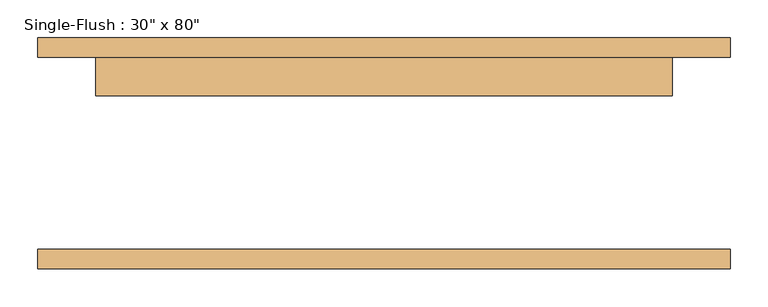
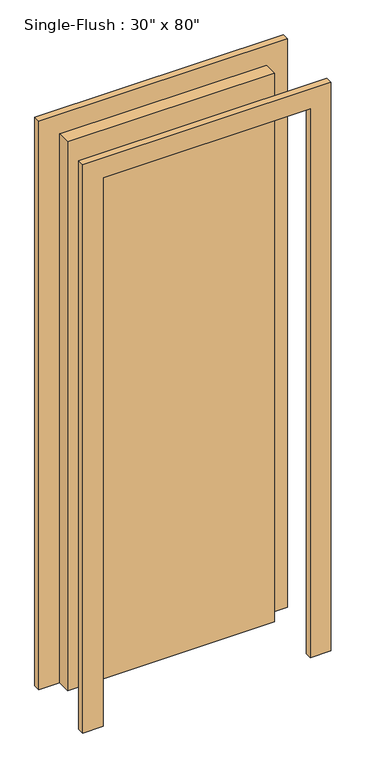
"""IFC4 building model written with IfcOpenShell, lengths in millimetres: door geometry."""

from ifc_helpers import new_model, si_unit, frame, origin, origin_with_axes, place, context, project, spatial, polyline, outline, extrude, source, transform, mapped, element, save


def door_bfeef022(model_context):
    return source(origin(), model_context, "Body", "SweptSolid", [
        extrude(outline(polyline([(2209.8, -457.2), (0.0, -457.2), (0.0, -381.0), (2133.6, -381.0), (2133.6, 381.0), (0.0, 381.0), (0.0, 457.2), (2209.8, 457.2), (2209.8, -457.2)])), frame((0.0, 127.0, 0.0), z_axis=(0.0, 1.0, 0.0), x_axis=(0.0, 0.0, 1.0)), (0.0, 0.0, 1.0), 25.4),
        extrude(outline(polyline([(2209.8, 457.2), (2209.8, -457.2), (0.0, -457.2), (0.0, -381.0), (2133.6, -381.0), (2133.6, 381.0), (0.0, 381.0), (0.0, 457.2), (2209.8, 457.2)])), frame((0.0, -152.4, 0.0), z_axis=(0.0, 1.0, 0.0), x_axis=(0.0, 0.0, 1.0)), (0.0, 0.0, 1.0), 25.4),
        extrude(outline(polyline([(381.0, 76.2), (-381.0, 76.2), (-381.0, 127.0), (381.0, 127.0), (381.0, 76.2)])), origin_with_axes(), (0.0, 0.0, 1.0), 2133.6),
    ])


if __name__ == "__main__":
    model = new_model("IFC4")
    model_context = context("Model", 3, world=origin())
    ifc_project = project(units=[si_unit("LENGTHUNIT", "METRE", prefix="MILLI")], contexts=[model_context])
    site = spatial("IfcSite", under=ifc_project)
    building = spatial("IfcBuilding", under=site)
    placement = place(None, origin())
    door_shape = door_bfeef022(model_context)
    element("IfcDoor", 1, ObjectType="Single-Flush : 30\" x 80\"", at=placement, inside=building, context=model_context, shape_type="MappedRepresentation", body=[
        mapped(door_shape, transform((0.0, 0.0, 0.0), x_axis=(1.0, 0.0, 0.0), y_axis=(0.0, 1.0, 0.0), z_axis=(0.0, 0.0, 1.0))),
    ])
    save(model, "model.ifc")

# Revit data of these elements
# Type "Single-Flush : 30\" x 80\""
#   Type Mark = "5"
#   Construction Type Id = "MDOOR"
#   Assembly Code = "C1020"
#   Analytic Construction = "Metal"
#   Thickness = 0' - 2"
#   Heat Transfer Coefficient (U) = 0.651978 BTU/(h·ft²·°F)
#   Height = 7' - 0"
#   Trim Projection Ext = 0' - 1"
#   Trim Projection Int = 0' - 1"
#   Trim Width = 0' - 3"
#   Width = 2' - 6"
#   Define Thermal Properties by = 1
#   Define Thermal Properties by = 1
#   Door Material = Door - Panel
#   Frame Material = Door - Frame
#   Visual Light Transmittance = 0
#   Solar Heat Gain Coefficient = 0
#   Function = (empty or 0)
#   Wall Closure = (empty or 0)
# Element 1 (IfcDoor, "Single-Flush : 30\" x 80\"")
#   Materials on its faces: "Door - Frame", "Door - Panel"
# Materials
#   "Door - Panel": class "Wood", colour RGB 210 159 95, transparency 0, Cost = 0
#   "Door - Frame": colour RGB 118 70 51, transparency 0, Cost = 0
